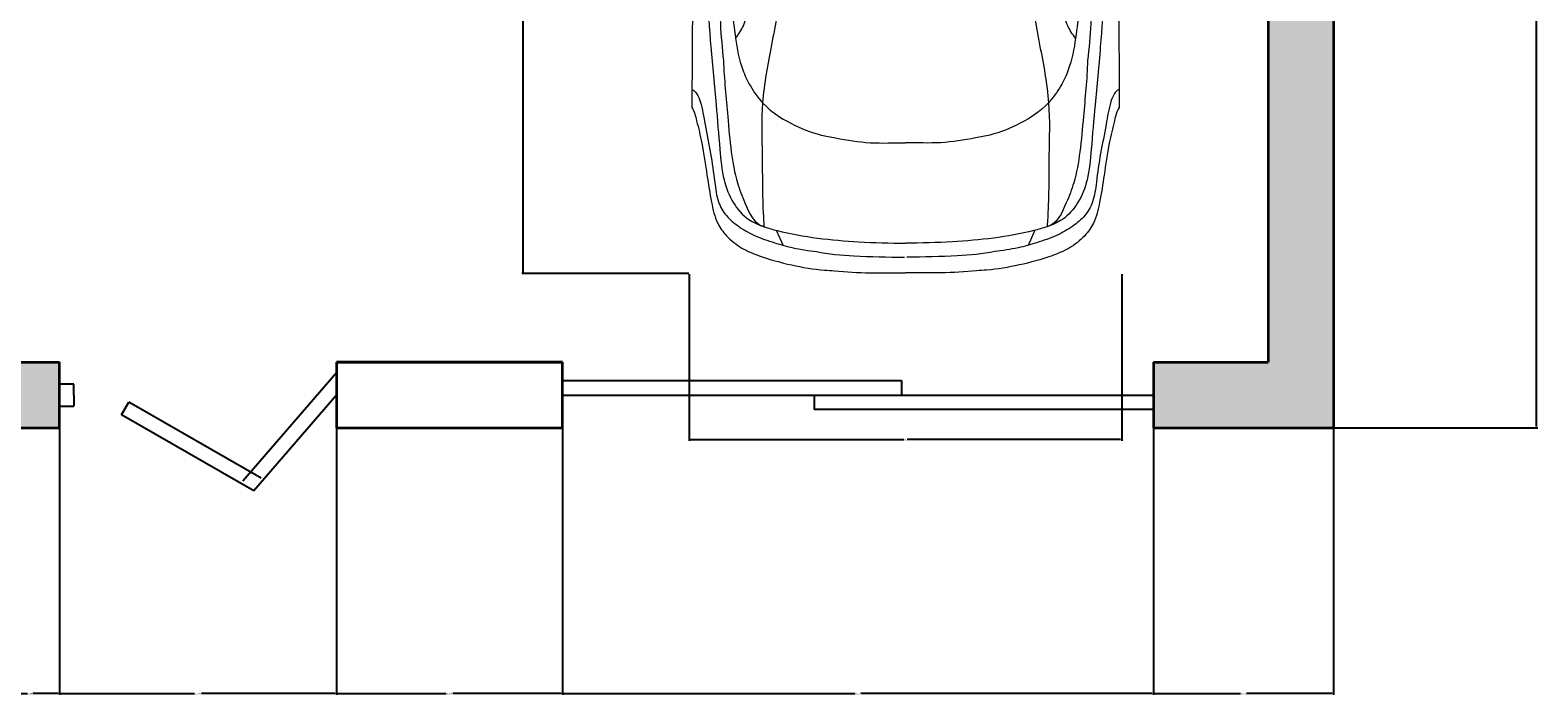
# Model space of a CAD drawing. Units: inches. Extents: x 1752 to 2227, y 6273 to 6884.
# Tile 2 of 6: x 2020 to 2227, y 6273 to 6365. Entities that reach past the tile are written whole.
import ezdxf

# ---------------------------------------------------------------- set-up
doc = ezdxf.new("R2010")
doc.units = ezdxf.units.IN
doc.header["$MEASUREMENT"] = 0
for name, color, linetype, lineweight in [('A-ANNO-DIMS', 2, 'Continuous', 18), ('A-DOOR-GATE', 3, 'Continuous', 25), ('A-EQPM-VEHI', 9, 'Continuous', 13), ('A-WALL', 7, 'Continuous', 35)]:
    doc.layers.add(name, color=color, linetype=linetype, lineweight=lineweight)
doc.layers.add('A-WALL-PATT', color=32, linetype='Continuous', lineweight=13, true_color=0xcd6928)
doc.styles.get("Standard").update_dxf_attribs({"font": 'arial.ttf'})
doc.dimstyles.get("Standard").update_dxf_attribs({"dimtxt": 0.18, "dimasz": 0.18, "dimexe": 0.18, "dimexo": 0.0625, "dimgap": 0.09, "dimtad": 0, "dimtih": 1, "dimtoh": 1, "dimdec": 4, "dimzin": 0, "dimdsep": 46, "dimtxsty": 'Standard', "dimcen": 0.09, "dimadec": 0, "dimazin": 0, "dimtfac": 1, "dimtdec": 4, "dimtofl": 0, "dimtmove": 0, "dimatfit": 3, "dimfxl": 1, "dimtolj": 1, "dimtzin": 0, "dimarcsym": 0})

# ---------------------------------------------------------------- blocks, each defined once
blk = doc.blocks.new('A$C242571DA')
for p, q in [((1714.3, 1732.5), (3817.1, 1739.9)), ((4315.2, 1398), (4377.3, 1370.5)), ((4315.2, 348.7), (4377.3, 376.3)), ((1714.3, 14.2), (3817.1, 6.9))]:
    blk.add_line(p, q)
for points, knots in [([(3745.3, 1736.8), (3748.5, 1730.1), (3764.2, 1717.1), (3811.5, 1698.6), (3894.7, 1686.7), (4002.9, 1663.2), (4107.9, 1648.7), (4195.8, 1638.3), (4258.6, 1603.2), (4302.1, 1549.7), (4339.9, 1483.8), (4365.2, 1407.6), (4389.6, 1324.4), (4397.9, 1266.9), (4401.8, 1235.2)], [0, 0, 0, 0, 0.0219205, 0.0572122, 0.1522539, 0.2718866, 0.3894011, 0.4710097, 0.5346344, 0.5986698, 0.6733118, 0.758696, 0.8351341, 0.9293726, 0.9293726, 0.9293726, 0.9293726]), ([(3817.1, 1739.9), (3833.2, 1729.7), (3882.9, 1718.2), (3973.3, 1695.2), (4085.1, 1680.5), (4193.8, 1662.8), (4280.6, 1644.3), (4343.9, 1598.1), (4390, 1540.3), (4427.4, 1448.7), (4457.8, 1336.6), (4475.7, 1233.4), (4478.4, 1175.1), (4479.3, 1161.6)], [0, 0, 0, 0, 0.056668, 0.14946, 0.28161, 0.392935, 0.481686, 0.542967, 0.622845, 0.69797, 0.833643, 0.965665, 1.00577, 1.00577, 1.00577, 1.00577]), ([(2695.2, 1655.3), (2829.9, 1655.3), (3041.2, 1651.4), (3351.3, 1630.7), (3527.5, 1623.2), (3626.6, 1612)], [0, 0, 0, 0, 0.4042759, 0.6333827, 0.9326252, 0.9326252, 0.9326252, 0.9326252]), ([(2984.7, 1695.8), (3051, 1695.6), (3172.1, 1691.3), (3367.4, 1677.6), (3575.2, 1664.3), (3788.2, 1643.6), (3968, 1628.1), (4103.8, 1616.8), (4203.6, 1578.1), (4271.8, 1519.5), (4300.6, 1452.1), (4341.7, 1305.3), (4361.8, 1111.2), (4367.5, 936.8), (4367.5, 873.4)], [0, 0, 0, 0, 0.198873, 0.363323, 0.587433, 0.823543, 1.004622, 1.129816, 1.230113, 1.320655, 1.388577, 1.443334, 1.771447, 1.958652, 1.958652, 1.958652, 1.958652]), ([(3535.9, 1563.1), (3520.1, 1550.9), (3484.4, 1526.1), (3408.2, 1510.9), (3323.4, 1473.1), (3207.9, 1445), (3072.6, 1422.2), (2866.9, 1404.6), (2626.4, 1412.9), (2396.7, 1410.8), (2200.9, 1416.9), (2001.3, 1438.2), (1732.1, 1525.9), (1527.9, 1578.9), (1407.5, 1610.7)], [0, 0, 0, 0, 0.05975, 0.126928, 0.230034, 0.336675, 0.482225, 0.641324, 0.954906, 1.203173, 1.330375, 1.542773, 1.802261, 2.175545, 2.175545, 2.175545, 2.175545]), ([(2861.6, 1607.5), (2921.1, 1607.3), (3047.2, 1600.8), (3191.4, 1602), (3356.6, 1584.1), (3498.3, 1570.6), (3623.2, 1549.4), (3664.1, 1533.3)], [0, 0, 0, 0, 0.1783018, 0.3787173, 0.431954, 0.6762374, 0.8077184, 0.8077184, 0.8077184, 0.8077184]), ([(3626.6, 1612), (3702.5, 1609.1), (3826.2, 1596.8), (3991.4, 1583.2), (4111.7, 1562.4), (4212.2, 1522.7), (4290.4, 1488), (4300.7, 1447.5)], [0, 0, 0, 0, 0.2277977, 0.3719478, 0.4996814, 0.5863441, 0.709615, 0.709615, 0.709615, 0.709615]), ([(3664.1, 1533.3), (3687, 1526), (3734.8, 1502.3), (3816.7, 1444.8), (3884.1, 1342.9), (3925.1, 1239.9), (3937.3, 1177), (3940.4, 1157.6)], [0, 0, 0, 0, 0.0720749, 0.1581284, 0.2958089, 0.4262456, 0.4842292, 0.4842292, 0.4842292, 0.4842292]), ([(1909.8, 1424.9), (1933.5, 1418.7), (1995.6, 1407.6), (2094.4, 1385.8), (2211.8, 1377.1), (2419, 1366.9), (2704.7, 1366.5), (3032.7, 1354.2), (3316.2, 1371), (3558.7, 1415.9), (3789.1, 1461.7), (4028.9, 1452.9), (4196.2, 1455.2), (4292.7, 1447.9), (4300.7, 1447.5)], [0, 0, 0, 0, 0.073325, 0.188896, 0.303039, 0.425821, 0.811242, 1.159737, 1.41058, 1.660623, 1.899627, 2.11145, 2.377727, 2.401703, 2.401703, 2.401703, 2.401703]), ([(4401.8, 1235.2), (4411.9, 1185.3), (4421.6, 1065.8), (4424.1, 946.5), (4424.1, 878)], [0, 0, 0, 0, 0.1502861, 0.3522699, 0.3522699, 0.3522699, 0.3522699]), ([(3940.4, 1157.6), (3949.9, 1111), (3964.3, 1016.4), (3960.5, 921), (3959.8, 873.4)], [0, 0, 0, 0, 0.140379, 0.2808468, 0.2808468, 0.2808468, 0.2808468]), ([(2984.7, 51), (3051, 51.1), (3172.1, 55.5), (3367.4, 69.2), (3575.2, 82.5), (3788.2, 103.1), (3968, 118.7), (4103.8, 130), (4203.6, 168.6), (4271.8, 227.3), (4300.6, 294.7), (4341.7, 441.5), (4361.8, 635.5), (4367.5, 809.9), (4367.5, 873.4)], [0, 0, 0, 0, 0.198873, 0.363323, 0.587433, 0.823543, 1.004622, 1.129816, 1.230113, 1.320655, 1.388577, 1.443334, 1.771447, 1.958652, 1.958652, 1.958652, 1.958652]), ([(3940.4, 589.1), (3949.9, 635.7), (3964.3, 730.4), (3960.5, 825.8), (3959.8, 873.4)], [0, 0, 0, 0, 0.140379, 0.2808468, 0.2808468, 0.2808468, 0.2808468]), ([(4401.8, 511.5), (4411.9, 561.5), (4421.6, 681), (4424.1, 800.3), (4424.1, 868.8)], [0, 0, 0, 0, 0.1502861, 0.3522699, 0.3522699, 0.3522699, 0.3522699]), ([(3664.1, 213.5), (3687, 220.8), (3734.8, 244.4), (3816.7, 302), (3884.1, 403.8), (3925.1, 506.9), (3937.3, 569.7), (3940.4, 589.1)], [0, 0, 0, 0, 0.0720749, 0.1581284, 0.2958089, 0.4262456, 0.4842292, 0.4842292, 0.4842292, 0.4842292]), ([(3817.1, 6.9), (3833.2, 17), (3882.9, 28.6), (3973.3, 51.5), (4085.1, 66.3), (4193.8, 84), (4280.6, 102.4), (4343.9, 148.6), (4390, 206.4), (4427.4, 298), (4457.8, 410.1), (4475.7, 513.3), (4478.4, 571.6), (4479.3, 585.2)], [0, 0, 0, 0, 0.056668, 0.14946, 0.28161, 0.392935, 0.481686, 0.542967, 0.622845, 0.69797, 0.833643, 0.965665, 1.00577, 1.00577, 1.00577, 1.00577]), ([(3745.3, 10), (3748.5, 16.7), (3764.2, 29.7), (3811.5, 48.1), (3894.7, 60.1), (4002.9, 83.6), (4107.9, 98), (4195.8, 108.4), (4258.6, 143.5), (4302.1, 197), (4339.9, 262.9), (4365.2, 339.2), (4389.6, 422.4), (4397.9, 479.8), (4401.8, 511.5)], [0, 0, 0, 0, 0.0219205, 0.0572122, 0.1522539, 0.2718866, 0.3894011, 0.4710097, 0.5346344, 0.5986698, 0.6733118, 0.758696, 0.8351341, 0.9293726, 0.9293726, 0.9293726, 0.9293726]), ([(1909.8, 321.9), (1933.5, 328.1), (1995.6, 339.2), (2094.4, 361), (2211.8, 369.6), (2419, 379.8), (2704.7, 380.3), (3032.7, 392.6), (3316.2, 375.8), (3558.7, 330.9), (3789.1, 285.1), (4028.9, 293.9), (4196.2, 291.5), (4292.7, 298.8), (4300.7, 299.2)], [0, 0, 0, 0, 0.073325, 0.188896, 0.303039, 0.425821, 0.811242, 1.159737, 1.41058, 1.660623, 1.899627, 2.11145, 2.377727, 2.401703, 2.401703, 2.401703, 2.401703]), ([(3535.9, 183.7), (3520.1, 195.9), (3484.4, 220.6), (3408.2, 235.8), (3323.4, 273.7), (3207.9, 301.8), (3072.6, 324.6), (2866.9, 342.1), (2626.4, 333.8), (2396.7, 335.9), (2200.9, 329.9), (2001.3, 308.6), (1732.1, 220.8), (1527.9, 167.8), (1407.5, 136)], [0, 0, 0, 0, 0.05975, 0.126928, 0.230034, 0.336675, 0.482225, 0.641324, 0.954906, 1.203173, 1.330375, 1.542773, 1.802261, 2.175545, 2.175545, 2.175545, 2.175545]), ([(3626.6, 134.7), (3702.5, 137.7), (3826.2, 149.9), (3991.4, 163.5), (4111.7, 184.4), (4212.2, 224.1), (4290.4, 258.8), (4300.7, 299.2)], [0, 0, 0, 0, 0.2277977, 0.3719478, 0.4996814, 0.5863441, 0.709615, 0.709615, 0.709615, 0.709615]), ([(2861.6, 139.2), (2921.1, 139.4), (3047.2, 146), (3191.4, 144.8), (3356.6, 162.6), (3498.3, 176.1), (3623.2, 197.4), (3664.1, 213.5)], [0, 0, 0, 0, 0.1783018, 0.3787173, 0.431954, 0.6762374, 0.8077184, 0.8077184, 0.8077184, 0.8077184]), ([(2695.2, 91.4), (2829.9, 91.5), (3041.2, 95.4), (3351.3, 116.1), (3527.5, 123.5), (3626.6, 134.7)], [0, 0, 0, 0, 0.4042759, 0.6333827, 0.9326252, 0.9326252, 0.9326252, 0.9326252])]:
    blk.add_open_spline(points, degree=3, knots=knots)
for points in [[(4479.3, 1161.6), (4491, 1066.2), (4488, 969.5), (4488, 873.4)], [(4479.3, 585.2), (4491, 680.6), (4488, 777.3), (4488, 873.4)]]:
    blk.add_open_spline(points, degree=3)
blk = doc.blocks.new('*D38')
at = {"layer": 'A-ANNO-DIMS', "color": 0, "lineweight": -2, "transparency": 16777216}
for p, q in [((2110.11, 6483.13), (2087.19, 6483.13)), ((2087.37, 6482.95), (2087.37, 6407.29)), ((2087.37, 6331.28), (2087.37, 6406.93)), ((2110.11, 6331.1), (2087.19, 6331.1))]:
    blk.add_line(p, q, dxfattribs=at)
at = {"layer": 'A-ANNO-DIMS', "color": 0, "transparency": 16777216}
for points in [[(2087.34, 6482.95), (2087.4, 6482.95), (2087.37, 6483.13)], [(2087.34, 6331.28), (2087.4, 6331.28), (2087.37, 6331.1)]]:
    blk.add_solid(points, dxfattribs=at)
at = {"layer": 'Defpoints', "color": 0, "transparency": 16777216}
for p in [(2110.17, 6483.13), (2087.37, 6331.1), (2110.17, 6331.1)]:
    blk.add_point(p, dxfattribs=at)
at = {"layer": 'A-ANNO-DIMS', "color": 0, "transparency": 16777216, "insert": (2087.37, 6407.11), "char_height": 0.18, "attachment_point": 5}
blk.add_mtext('\\A1;CAR 152', dxfattribs=at)
blk = doc.blocks.new('*D39')
at = {"layer": 'A-ANNO-DIMS', "color": 0, "lineweight": -2, "transparency": 16777216}
for p, q in [((2110.17, 6331.03), (2110.17, 6308.11)), ((2169.58, 6331.03), (2169.58, 6308.11)), ((2110.35, 6308.29), (2139.66, 6308.29)), ((2169.4, 6308.29), (2140.09, 6308.29))]:
    blk.add_line(p, q, dxfattribs=at)
at = {"layer": 'A-ANNO-DIMS', "color": 0, "transparency": 16777216}
for points in [[(2110.35, 6308.32), (2110.35, 6308.26), (2110.17, 6308.29)], [(2169.4, 6308.32), (2169.4, 6308.26), (2169.58, 6308.29)]]:
    blk.add_solid(points, dxfattribs=at)
at = {"layer": 'Defpoints', "color": 0, "transparency": 16777216}
for p in [(2110.17, 6331.1), (2169.58, 6331.1), (2169.58, 6308.29)]:
    blk.add_point(p, dxfattribs=at)
at = {"layer": 'A-ANNO-DIMS', "color": 0, "transparency": 16777216, "insert": (2139.88, 6308.29), "char_height": 0.18, "attachment_point": 5}
blk.add_mtext('\\A1;59', dxfattribs=at)
blk = doc.blocks.new('*D42')
at = {"layer": 'A-ANNO-DIMS', "color": 0, "lineweight": -2, "transparency": 16777216}
for p, q in [((2189.71, 6501.91), (2226.68, 6501.91)), ((2226.5, 6501.73), (2226.5, 6406.1)), ((2226.5, 6310.09), (2226.5, 6405.73)), ((2198.71, 6309.91), (2226.68, 6309.91))]:
    blk.add_line(p, q, dxfattribs=at)
at = {"layer": 'A-ANNO-DIMS', "color": 0, "transparency": 16777216}
for points in [[(2226.47, 6501.73), (2226.53, 6501.73), (2226.5, 6501.91)], [(2226.47, 6310.09), (2226.53, 6310.09), (2226.5, 6309.91)]]:
    blk.add_solid(points, dxfattribs=at)
at = {"layer": 'Defpoints', "color": 0, "transparency": 16777216}
for p in [(2189.65, 6501.91), (2226.5, 6501.91), (2198.65, 6309.91)]:
    blk.add_point(p, dxfattribs=at)
at = {"layer": 'A-ANNO-DIMS', "color": 0, "transparency": 16777216, "insert": (2226.5, 6405.91), "char_height": 0.18, "attachment_point": 5}
blk.add_mtext('\\A1;192', dxfattribs=at)
blk = doc.blocks.new('*D50')
at = {"layer": 'A-ANNO-DIMS', "color": 0, "lineweight": -2, "transparency": 16777216}
for p, q in [((2015.65, 6375.85), (2015.65, 6273.23)), ((2023.68, 6309.85), (2023.68, 6273.23)), ((2015.83, 6273.41), (2019.29, 6273.41)), ((2023.5, 6273.41), (2020.04, 6273.41))]:
    blk.add_line(p, q, dxfattribs=at)
at = {"layer": 'A-ANNO-DIMS', "color": 0, "transparency": 16777216}
for points in [[(2015.83, 6273.44), (2015.83, 6273.38), (2015.65, 6273.41)], [(2023.5, 6273.44), (2023.5, 6273.38), (2023.68, 6273.41)]]:
    blk.add_solid(points, dxfattribs=at)
at = {"layer": 'Defpoints', "color": 0, "transparency": 16777216}
for p in [(2015.65, 6375.91), (2023.68, 6309.91), (2023.68, 6273.41)]:
    blk.add_point(p, dxfattribs=at)
at = {"layer": 'A-ANNO-DIMS', "color": 0, "transparency": 16777216, "insert": (2019.66, 6273.41), "char_height": 0.18, "attachment_point": 5}
blk.add_mtext('\\A1;8.031', dxfattribs=at)
blk = doc.blocks.new('*D51')
at = {"layer": 'A-ANNO-DIMS', "color": 0, "lineweight": -2, "transparency": 16777216}
for p, q in [((2023.68, 6309.85), (2023.68, 6273.23)), ((2061.74, 6309.85), (2061.74, 6273.23)), ((2023.86, 6273.41), (2042.25, 6273.41)), ((2061.56, 6273.41), (2043.18, 6273.41))]:
    blk.add_line(p, q, dxfattribs=at)
at = {"layer": 'A-ANNO-DIMS', "color": 0, "transparency": 16777216}
for points in [[(2023.86, 6273.44), (2023.86, 6273.38), (2023.68, 6273.41)], [(2061.56, 6273.44), (2061.56, 6273.38), (2061.74, 6273.41)]]:
    blk.add_solid(points, dxfattribs=at)
at = {"layer": 'Defpoints', "color": 0, "transparency": 16777216}
for p in [(2023.68, 6309.91), (2061.74, 6309.91), (2061.74, 6273.41)]:
    blk.add_point(p, dxfattribs=at)
at = {"layer": 'A-ANNO-DIMS', "color": 0, "transparency": 16777216, "insert": (2042.71, 6273.41), "char_height": 0.18, "attachment_point": 5}
blk.add_mtext('\\A1;38.065', dxfattribs=at)
blk = doc.blocks.new('*D52')
at = {"layer": 'A-ANNO-DIMS', "color": 0, "lineweight": -2, "transparency": 16777216}
for p, q in [((2061.74, 6309.85), (2061.74, 6273.23)), ((2092.75, 6309.85), (2092.75, 6273.23)), ((2061.92, 6273.41), (2076.78, 6273.41)), ((2092.57, 6273.41), (2077.71, 6273.41))]:
    blk.add_line(p, q, dxfattribs=at)
at = {"layer": 'A-ANNO-DIMS', "color": 0, "transparency": 16777216}
for points in [[(2061.92, 6273.44), (2061.92, 6273.38), (2061.74, 6273.41)], [(2092.57, 6273.44), (2092.57, 6273.38), (2092.75, 6273.41)]]:
    blk.add_solid(points, dxfattribs=at)
at = {"layer": 'Defpoints', "color": 0, "transparency": 16777216}
for p in [(2061.74, 6309.91), (2092.75, 6309.91), (2092.75, 6273.41)]:
    blk.add_point(p, dxfattribs=at)
at = {"layer": 'A-ANNO-DIMS', "color": 0, "transparency": 16777216, "insert": (2077.25, 6273.41), "char_height": 0.18, "attachment_point": 5}
blk.add_mtext('\\A1;31.006', dxfattribs=at)
blk = doc.blocks.new('*D53')
at = {"layer": 'A-ANNO-DIMS', "color": 0, "lineweight": -2, "transparency": 16777216}
for p, q in [((2092.75, 6309.85), (2092.75, 6273.23)), ((2173.93, 6309.85), (2173.93, 6273.23)), ((2092.93, 6273.41), (2132.94, 6273.41)), ((2173.75, 6273.41), (2133.73, 6273.41))]:
    blk.add_line(p, q, dxfattribs=at)
at = {"layer": 'A-ANNO-DIMS', "color": 0, "transparency": 16777216}
for points in [[(2092.93, 6273.44), (2092.93, 6273.38), (2092.75, 6273.41)], [(2173.75, 6273.44), (2173.75, 6273.38), (2173.93, 6273.41)]]:
    blk.add_solid(points, dxfattribs=at)
at = {"layer": 'Defpoints', "color": 0, "transparency": 16777216}
for p in [(2092.75, 6309.91), (2173.93, 6309.91), (2173.93, 6273.41)]:
    blk.add_point(p, dxfattribs=at)
at = {"layer": 'A-ANNO-DIMS', "color": 0, "transparency": 16777216, "insert": (2133.34, 6273.41), "char_height": 0.18, "attachment_point": 5}
blk.add_mtext('\\A1;81.18', dxfattribs=at)
blk = doc.blocks.new('*D54')
at = {"layer": 'A-ANNO-DIMS', "color": 0, "lineweight": -2, "transparency": 16777216}
for p, q in [((2173.93, 6309.85), (2173.93, 6273.23)), ((2198.65, 6309.85), (2198.65, 6273.23)), ((2174.11, 6273.41), (2185.89, 6273.41)), ((2198.47, 6273.41), (2186.68, 6273.41))]:
    blk.add_line(p, q, dxfattribs=at)
at = {"layer": 'A-ANNO-DIMS', "color": 0, "transparency": 16777216}
for points in [[(2174.11, 6273.44), (2174.11, 6273.38), (2173.93, 6273.41)], [(2198.47, 6273.44), (2198.47, 6273.38), (2198.65, 6273.41)]]:
    blk.add_solid(points, dxfattribs=at)
at = {"layer": 'Defpoints', "color": 0, "transparency": 16777216}
for p in [(2173.93, 6309.91), (2198.65, 6309.91), (2198.65, 6273.41)]:
    blk.add_point(p, dxfattribs=at)
at = {"layer": 'A-ANNO-DIMS', "color": 0, "transparency": 16777216, "insert": (2186.29, 6273.41), "char_height": 0.18, "attachment_point": 5}
blk.add_mtext('\\A1;24.72', dxfattribs=at)

msp = doc.modelspace()

# ---------------------------------------------------------------- hatches: boundary and pattern name
at = {"layer": 'A-WALL-PATT'}
h = msp.add_hatch(color=256, dxfattribs=at)
h.dxf.hatch_style = 1
h.paths.add_polyline_path([(2198.6473, 6855.914), (1780.1473, 6855.914), (1780.1473, 6309.914), (1824.3861, 6309.914), (1824.3861, 6318.914), (1789.1473, 6318.914), (1789.1473, 6501.914), (1790.1473, 6501.914), (1790.1473, 6510.914), (1789.1473, 6510.914), (1789.1473, 6570.914), (1838.6473, 6570.914), (1838.6473, 6510.914), (1822.1473, 6510.914), (1822.1473, 6501.914), (1921.1473, 6501.914), (1921.1473, 6498.914), (1930.1473, 6498.914), (1930.1473, 6501.914), (1930.1473, 6510.914), (1847.6473, 6510.914), (1847.6473, 6585.039), (1838.6473, 6585.039), (1838.6473, 6575.414), (1789.1473, 6575.414), (1789.1473, 6705.914), (1795.2039, 6705.914), (1795.2039, 6714.914), (1789.1473, 6714.914), (1789.1473, 6846.914), (1984.1473, 6846.914), (1984.1473, 6714.914), (1977.8419, 6714.914), (1977.8419, 6705.914), (1984.1473, 6705.914), (1984.1473, 6651.914), (1977.6147, 6651.914), (1977.6147, 6642.914), (1996.1473, 6642.914), (1996.1473, 6651.914), (1993.1473, 6651.914), (1993.1473, 6846.914), (2125.1473, 6846.914), (2125.1473, 6840.4779), (2129.6473, 6840.4779), (2129.6473, 6846.914), (2189.6473, 6846.914), (2189.6473, 6798.914), (2162.6473, 6798.914), (2162.6473, 6794.414), (2189.6473, 6794.414), (2189.6473, 6710.414), (2175.6868, 6710.414), (2175.6868, 6705.914), (2189.6473, 6705.914), (2189.6473, 6651.914), (2164.6473, 6651.914), (2164.6473, 6642.914), (2189.6473, 6642.914), (2189.6473, 6510.914), (2166.7624, 6510.914), (2166.7624, 6501.914), (2189.6473, 6501.914), (2189.6473, 6318.914), (2173.9269, 6318.914), (2173.9269, 6309.914), (2198.6473, 6309.914)])
h.paths.add_polyline_path([(2023.6785, 6318.914), (1930.1473, 6318.914), (1930.1473, 6321.914), (1921.1473, 6321.914), (1921.1473, 6318.914), (1872.3861, 6318.914), (1872.3861, 6309.914), (2023.6785, 6309.914)], flags=17)
h.paths.add_polyline_path([(2092.7496, 6318.914), (2061.7431, 6318.914), (2061.7431, 6309.914), (2092.7496, 6309.914)], flags=0)
h.paths.add_polyline_path([(1947.0033, 6375.914), (1930.1473, 6375.914), (1930.1473, 6462.914), (1921.1473, 6462.914), (1921.1473, 6357.914), (1930.1473, 6357.914), (1930.1473, 6366.914), (1947.0033, 6366.914)], flags=17)
h.paths.add_polyline_path([(2024.6473, 6432.914), (2015.6473, 6432.914), (2015.6473, 6375.914), (1995.0033, 6375.914), (1995.0033, 6366.914), (2024.6473, 6366.914)], flags=17)
h.paths.add_polyline_path([(2030.6473, 6441.914), (2024.6473, 6441.914), (2024.6473, 6510.914), (2015.6473, 6510.914), (2015.6473, 6432.914), (2024.6473, 6432.914), (2030.6473, 6432.914)], flags=17)
h.paths.add_polyline_path([(2093.6473, 6501.914), (2118.7624, 6501.914), (2118.7624, 6510.914), (2093.6473, 6510.914), (2093.6473, 6603.914), (2084.6473, 6603.914), (2084.6473, 6441.914), (2078.6473, 6441.914), (2078.6473, 6432.914), (2093.6473, 6432.914)], flags=17)
h.paths.add_polyline_path([(2132.6473, 6651.914), (2129.6473, 6651.914), (2129.6473, 6705.914), (2139.6868, 6705.914), (2139.6868, 6710.414), (2129.6473, 6710.414), (2129.6473, 6794.414), (2130.6473, 6794.414), (2130.6473, 6798.914), (2129.6473, 6798.914), (2129.6473, 6804.4779), (2125.1473, 6804.4779), (2125.1473, 6651.914), (2032.1473, 6651.914), (2032.1473, 6642.914), (2084.6473, 6642.914), (2084.6473, 6639.914), (2093.6473, 6639.914), (2093.6473, 6642.914), (2132.6473, 6642.914)], flags=17)
h.paths.add_polyline_path([(1929.6147, 6651.914), (1924.1473, 6651.914), (1924.1473, 6705.914), (1941.8419, 6705.914), (1941.8419, 6714.914), (1911.8299, 6714.914), (1911.8299, 6705.914), (1919.6473, 6705.914), (1919.6473, 6651.914), (1847.6473, 6651.914), (1847.6473, 6662.4635), (1838.6473, 6662.4635), (1838.6473, 6621.039), (1847.6473, 6621.039), (1847.6473, 6642.914), (1929.6147, 6642.914)], flags=17)
h.paths.add_polyline_path([(1879.8299, 6714.914), (1831.2039, 6714.914), (1831.2039, 6705.914), (1838.6473, 6705.914), (1838.6473, 6698.4635), (1847.6473, 6698.4635), (1847.6473, 6705.914), (1879.8299, 6705.914)], flags=17)

# ---------------------------------------------------------------- linework, layer by layer
at = {"layer": 'A-DOOR-GATE'}
for p, q in [((2061.7431, 6317.4756), (2048.8828, 6302.5704)), ((2025.6547, 6315.897), (2023.6785, 6315.897)), ((2023.6785, 6315.897), (2023.6785, 6312.897)), ((2025.6417, 6314.397), (2025.6547, 6315.897)), ((2092.7496, 6316.414), (2139.3382, 6316.414)), ((2139.3382, 6316.414), (2139.3382, 6314.414)), ((2023.6785, 6312.897), (2025.6417, 6312.897)), ((2025.6417, 6314.397), (2025.6417, 6312.897)), ((2032.2085, 6311.6874), (2033.2029, 6313.4226)), ((2051.3915, 6302.9991), (2033.2029, 6313.4226)), ((2061.7431, 6314.414), (2050.397, 6301.2639)), ((2092.7496, 6314.414), (2173.9269, 6314.414)), ((2127.3382, 6314.414), (2127.3382, 6312.414)), ((2050.397, 6301.2639), (2032.2085, 6311.6874)), ((2173.9269, 6312.414), (2127.3382, 6312.414))]:
    msp.add_line(p, q, dxfattribs=at)
at = {"layer": 'A-WALL'}
for p, q in [((2198.6473, 6855.914), (2198.6473, 6309.914)), ((2189.6473, 6501.914), (2189.6473, 6318.914)), ((1930.1473, 6318.914), (2023.6785, 6318.914)), ((2023.6785, 6309.914), (2023.6785, 6318.914)), ((2092.7496, 6318.914), (2061.7431, 6318.914)), ((2061.7431, 6318.914), (2061.7431, 6309.914)), ((2061.7431, 6318.914), (2092.7496, 6318.914)), ((2092.7496, 6309.914), (2092.7496, 6318.914)), ((2173.9269, 6318.914), (2173.9269, 6309.914)), ((2173.9269, 6318.914), (2189.6473, 6318.914)), ((1780.1473, 6309.914), (2023.6785, 6309.914)), ((2061.7431, 6309.914), (2092.7496, 6309.914)), ((2061.7431, 6309.914), (2092.7496, 6309.914)), ((2173.9269, 6309.914), (2198.6473, 6309.914))]:
    msp.add_line(p, q, dxfattribs=at)

# ---------------------------------------------------------------- block references
at = {"layer": 'A-EQPM-VEHI', "xscale": 0.0338519890313957, "yscale": 0.0338519890313957, "zscale": 0.0338519890313957, "rotation": 270}
msp.add_blockref('A$C242571DA', (2110.3102, 6483.126), dxfattribs=at)

# ---------------------------------------------------------------- dimensions: what is measured, and where the dimension line sits
at = {"layer": 'A-ANNO-DIMS'}
dim = msp.add_linear_dim(base=(2226.4973, 6501.914), p1=(2198.6473, 6309.914), p2=(2189.6473, 6501.914), angle=90, dimstyle='Standard', override={"dimdec": 0, "dimlfac": 1, "dimrnd": 0, "dimzin": 0, "dimdsep": 46, "dimlunit": 2}, dxfattribs=at)
dim.commit()
dim.dimension.update_dxf_attribs({"geometry": '*D42', "text_midpoint": (2226.4973, 6405.914)})
dim = msp.add_linear_dim(base=(2087.3665, 6331.095), p1=(2110.1711, 6483.126), p2=(2110.1711, 6331.095), angle=270, text='CAR <>', dimstyle='Standard', override={"dimdec": 0, "dimlfac": 1, "dimrnd": 0, "dimzin": 0, "dimdsep": 46, "dimlunit": 2}, dxfattribs=at)
dim.commit()
dim.dimension.update_dxf_attribs({"geometry": '*D38', "text_midpoint": (2087.3665, 6407.1105)})
for base, p1, p2, override, picture, middle in [((2023.6785, 6273.4139), (2015.6473, 6375.914), (2023.6785, 6309.914), {"dimdec": 3, "dimlfac": 1, "dimrnd": 0, "dimzin": 0, "dimdsep": 46, "dimlunit": 2}, '*D50', (2019.6629, 6273.4139)), ((2169.5806, 6308.2904), (2110.1711, 6331.095), (2169.5806, 6331.095), {"dimdec": 0, "dimlfac": 1, "dimrnd": 0, "dimzin": 0, "dimdsep": 46, "dimlunit": 2}, '*D39', (2139.8759, 6308.2904)), ((2061.7431, 6273.4139), (2023.6785, 6309.914), (2061.7431, 6309.914), {"dimdec": 3, "dimlfac": 1, "dimrnd": 0, "dimzin": 0, "dimdsep": 46, "dimlunit": 2}, '*D51', (2042.7108, 6273.4139)), ((2092.74956, 6273.41389), (2061.74314, 6309.91404), (2092.74956, 6309.91404), {"dimdec": 3, "dimlfac": 1, "dimrnd": 0, "dimzin": 0, "dimdsep": 46, "dimlunit": 2}, '*D52', (2077.24635, 6273.41389)), ((2173.9269, 6273.4139), (2092.7496, 6309.914), (2173.9269, 6309.914), {"dimdec": 2, "dimlfac": 1, "dimrnd": 0, "dimzin": 0, "dimdsep": 46, "dimlunit": 2}, '*D53', (2133.3382, 6273.4139)), ((2198.6473, 6273.4139), (2173.9269, 6309.914), (2198.6473, 6309.914), {"dimdec": 2, "dimlfac": 1, "dimrnd": 0, "dimzin": 0, "dimdsep": 46, "dimlunit": 2}, '*D54', (2186.2871, 6273.4139))]:
    dim = msp.add_linear_dim(base=base, p1=p1, p2=p2, dimstyle='Standard', override=override, dxfattribs=at)
    dim.commit()
    dim.dimension.update_dxf_attribs({"geometry": picture, "text_midpoint": middle})

doc.saveas('drawing.dxf')
